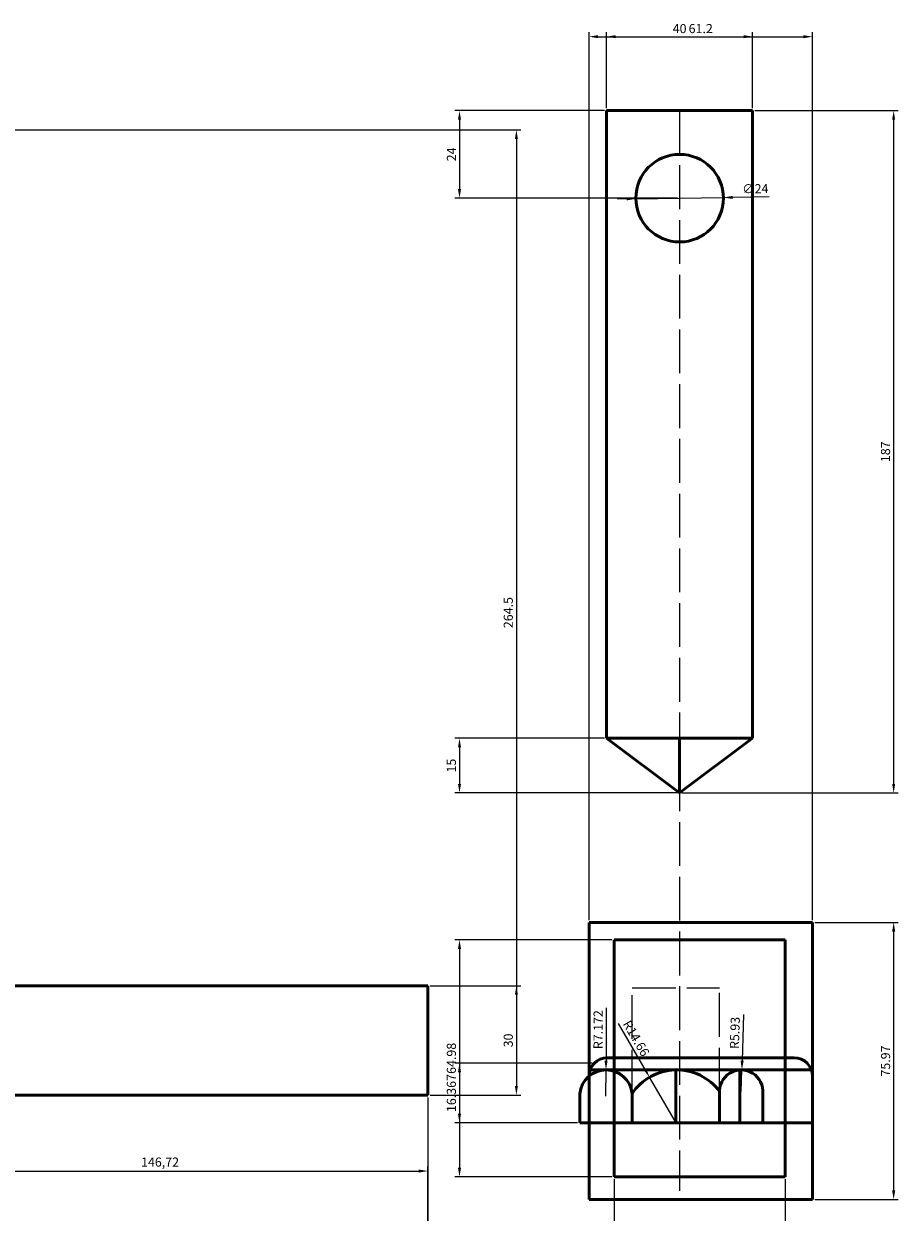
# Model space of a CAD drawing. Units: millimetres. Extents: x 921 to 2648, y 1390 to 2315.
# Tile 3 of 10: x 1184 to 1424, y 1882 to 2207. Entities that reach past the tile are written whole.
import ezdxf

# ---------------------------------------------------------------- set-up
doc = ezdxf.new("R2010")
doc.units = ezdxf.units.MM
doc.linetypes.add('ACAD_ISO02W100', pattern=[15, 12, -3])
for name, color, linetype, lineweight in [('M-DIMS', 2, 'Continuous', 25), ('M-HIDN', 4, 'ACAD_ISO02W100', 25), ('M-OUTL', 7, 'Continuous', 50)]:
    doc.layers.add(name, color=color, linetype=linetype, lineweight=lineweight)
doc.styles.get("Standard").update_dxf_attribs({"font": 'arial.ttf'})
doc.dimstyles.new('ISO-25', dxfattribs={"dimtxt": 2.5, "dimasz": 2.5, "dimexe": 1.25, "dimexo": 0.625, "dimtad": 1, "dimtxsty": 'Standard', "dimcen": 2.5, "dimadec": 0, "dimazin": 0, "dimtfac": 1, "dimtmove": 0, "dimatfit": 3, "dimfxl": 1, "dimarcsym": 0})

# ---------------------------------------------------------------- blocks, each defined once
blk = doc.blocks.new('*D18')
at = {"layer": 'Defpoints', "color": 0, "transparency": 16777216}
for p in [(1148.08, 1948.7), (1294.79, 1892.9), (1294.79, 1878.16)]:
    blk.add_point(p, dxfattribs=at)
at = {"layer": 'M-DIMS', "color": 0, "lineweight": -2, "transparency": 16777216}
for p, q in [((1148.08, 1948.07), (1148.08, 1891.65)), ((1150.58, 1892.9), (1292.29, 1892.9)), ((1294.79, 1878.78), (1294.79, 1894.15))]:
    blk.add_line(p, q, dxfattribs=at)
at = {"layer": 'M-DIMS', "color": 0, "transparency": 16777216}
for points in [[(1150.58, 1893.32), (1150.58, 1892.48), (1148.08, 1892.9)], [(1292.29, 1893.32), (1292.29, 1892.48), (1294.79, 1892.9)]]:
    blk.add_solid(points, dxfattribs=at)
at = {"layer": 'M-DIMS', "color": 0, "transparency": 16777216, "insert": (1221.43, 1895.03), "char_height": 2.5, "attachment_point": 5}
blk.add_mtext('146,72', dxfattribs=at)
blk = doc.blocks.new('*D24')
at = {"layer": 'Defpoints', "color": 0, "transparency": 16777216}
for p in [(1383.76, 2203.78), (1343.76, 2183.53), (1383.76, 2183.53)]:
    blk.add_point(p, dxfattribs=at)
at = {"layer": 'M-DIMS', "color": 0, "lineweight": -2, "transparency": 16777216}
for p, q in [((1343.76, 2184.15), (1343.76, 2205.03)), ((1346.26, 2203.78), (1381.26, 2203.78)), ((1383.76, 2184.15), (1383.76, 2205.03))]:
    blk.add_line(p, q, dxfattribs=at)
at = {"layer": 'M-DIMS', "color": 0, "transparency": 16777216}
for points in [[(1346.26, 2204.2), (1346.26, 2203.36), (1343.76, 2203.78)], [(1381.26, 2204.2), (1381.26, 2203.36), (1383.76, 2203.78)]]:
    blk.add_solid(points, dxfattribs=at)
at = {"layer": 'M-DIMS', "color": 0, "transparency": 16777216, "insert": (1363.76, 2205.68), "char_height": 2.5, "attachment_point": 5}
blk.add_mtext('40', dxfattribs=at)
blk = doc.blocks.new('*D25')
at = {"layer": 'Defpoints', "color": 0, "transparency": 16777216}
for p in [(1383.76, 2183.53), (1363.76, 1996.51), (1422.39, 1996.51)]:
    blk.add_point(p, dxfattribs=at)
at = {"layer": 'M-DIMS', "color": 0, "lineweight": -2, "transparency": 16777216}
for p, q in [((1384.39, 2183.53), (1423.64, 2183.53)), ((1422.39, 2181.03), (1422.39, 1999.01)), ((1364.39, 1996.51), (1423.64, 1996.51))]:
    blk.add_line(p, q, dxfattribs=at)
at = {"layer": 'M-DIMS', "color": 0, "transparency": 16777216}
for points in [[(1421.97, 2181.03), (1422.81, 2181.03), (1422.39, 2183.53)], [(1421.97, 1999.01), (1422.81, 1999.01), (1422.39, 1996.51)]]:
    blk.add_solid(points, dxfattribs=at)
at = {"layer": 'M-DIMS', "color": 0, "transparency": 16777216, "insert": (1420.49, 2090.02), "char_height": 2.5, "attachment_point": 5, "rotation": 90}
blk.add_mtext('187', dxfattribs=at)
blk = doc.blocks.new('*D45')
at = {"layer": 'Defpoints', "color": 0, "transparency": 16777216}
for p in [(1294.79, 1943.7), (1294.79, 1913.7), (1319.04, 1913.7)]:
    blk.add_point(p, dxfattribs=at)
at = {"layer": 'M-DIMS', "color": 0, "lineweight": -2, "transparency": 16777216}
for p, q in [((1295.42, 1943.7), (1320.29, 1943.7)), ((1319.04, 1941.2), (1319.04, 1916.2)), ((1295.42, 1913.7), (1320.29, 1913.7))]:
    blk.add_line(p, q, dxfattribs=at)
at = {"layer": 'M-DIMS', "color": 0, "transparency": 16777216}
for points in [[(1318.63, 1941.2), (1319.46, 1941.2), (1319.04, 1943.7)], [(1318.63, 1916.2), (1319.46, 1916.2), (1319.04, 1913.7)]]:
    blk.add_solid(points, dxfattribs=at)
at = {"layer": 'M-DIMS', "color": 0, "transparency": 16777216, "insert": (1317.14, 1928.7), "char_height": 2.5, "attachment_point": 5, "rotation": 90}
blk.add_mtext('30', dxfattribs=at)
blk = doc.blocks.new('*D46')
at = {"layer": 'Defpoints', "color": 0, "transparency": 16777216}
for p in [(1148.08, 2178.21), (1294.79, 1913.7), (1319.04, 1913.7)]:
    blk.add_point(p, dxfattribs=at)
at = {"layer": 'M-DIMS', "color": 0, "lineweight": -2, "transparency": 16777216}
for p, q in [((1148.7, 2178.21), (1320.29, 2178.21)), ((1319.04, 2175.71), (1319.04, 1916.2)), ((1295.42, 1913.7), (1320.29, 1913.7))]:
    blk.add_line(p, q, dxfattribs=at)
at = {"layer": 'M-DIMS', "color": 0, "transparency": 16777216}
for points in [[(1318.63, 2175.71), (1319.46, 2175.71), (1319.04, 2178.21)], [(1318.63, 1916.2), (1319.46, 1916.2), (1319.04, 1913.7)]]:
    blk.add_solid(points, dxfattribs=at)
at = {"layer": 'M-DIMS', "color": 0, "transparency": 16777216, "insert": (1317.14, 2045.95), "char_height": 2.5, "attachment_point": 5, "rotation": 90}
blk.add_mtext('264.5', dxfattribs=at)
blk = doc.blocks.new('*D49')
at = {"layer": 'Defpoints', "color": 0, "transparency": 16777216}
for p in [(950.61, 1913.7), (1294.79, 1913.7), (1294.79, 1705.98)]:
    blk.add_point(p, dxfattribs=at)
at = {"layer": 'M-DIMS', "color": 0, "lineweight": -2, "transparency": 16777216}
for p, q in [((950.61, 1913.07), (950.61, 1704.73)), ((1294.79, 1913.07), (1294.79, 1704.73)), ((953.11, 1705.98), (1292.29, 1705.98))]:
    blk.add_line(p, q, dxfattribs=at)
at = {"layer": 'M-DIMS', "color": 0, "transparency": 16777216}
for points in [[(953.11, 1706.4), (953.11, 1705.56), (950.61, 1705.98)], [(1292.29, 1706.4), (1292.29, 1705.56), (1294.79, 1705.98)]]:
    blk.add_solid(points, dxfattribs=at)
at = {"layer": 'M-DIMS', "color": 0, "transparency": 16777216, "insert": (1122.7, 1707.88), "char_height": 2.5, "attachment_point": 5}
blk.add_mtext('344.2', dxfattribs=at)
blk = doc.blocks.new('*D54')
at = {"layer": 'Defpoints', "color": 0, "transparency": 16777216}
for p in [(1343.76, 2183.53), (1303.46, 2159.53), (1363.76, 2159.53)]:
    blk.add_point(p, dxfattribs=at)
at = {"layer": 'M-DIMS', "color": 0, "lineweight": -2, "transparency": 16777216}
for p, q in [((1343.14, 2183.53), (1302.21, 2183.53)), ((1303.46, 2181.03), (1303.46, 2162.03)), ((1363.14, 2159.53), (1302.21, 2159.53))]:
    blk.add_line(p, q, dxfattribs=at)
at = {"layer": 'M-DIMS', "color": 0, "transparency": 16777216}
for points in [[(1303.04, 2181.03), (1303.88, 2181.03), (1303.46, 2183.53)], [(1303.04, 2162.03), (1303.88, 2162.03), (1303.46, 2159.53)]]:
    blk.add_solid(points, dxfattribs=at)
at = {"layer": 'M-DIMS', "color": 0, "transparency": 16777216, "insert": (1301.58, 2171.53), "char_height": 2.5, "attachment_point": 5, "rotation": 90}
blk.add_mtext('24', dxfattribs=at)
blk = doc.blocks.new('*D55')
at = {"layer": 'Defpoints', "color": 0, "transparency": 16777216}
for p in [(1343.76, 2011.51), (1303.46, 1996.51), (1363.76, 1996.51)]:
    blk.add_point(p, dxfattribs=at)
at = {"layer": 'M-DIMS', "color": 0, "lineweight": -2, "transparency": 16777216}
for p, q in [((1343.14, 2011.51), (1302.21, 2011.51)), ((1303.46, 2009.01), (1303.46, 1999.01)), ((1363.14, 1996.51), (1302.21, 1996.51))]:
    blk.add_line(p, q, dxfattribs=at)
at = {"layer": 'M-DIMS', "color": 0, "transparency": 16777216}
for points in [[(1303.04, 2009.01), (1303.88, 2009.01), (1303.46, 2011.51)], [(1303.04, 1999.01), (1303.88, 1999.01), (1303.46, 1996.51)]]:
    blk.add_solid(points, dxfattribs=at)
at = {"layer": 'M-DIMS', "color": 0, "transparency": 16777216, "insert": (1301.56, 2004.01), "char_height": 2.5, "attachment_point": 5, "rotation": 90}
blk.add_mtext('15', dxfattribs=at)
blk = doc.blocks.new('*D56')
at = {"layer": 'Defpoints', "color": 0, "transparency": 16777216}
for p in [(1400.14, 2203.78), (1338.94, 1961.04), (1400.14, 1961.04)]:
    blk.add_point(p, dxfattribs=at)
at = {"layer": 'M-DIMS', "color": 0, "lineweight": -2, "transparency": 16777216}
for p, q in [((1338.94, 1961.66), (1338.94, 2205.03)), ((1341.44, 2203.78), (1397.64, 2203.78)), ((1400.14, 1961.66), (1400.14, 2205.03))]:
    blk.add_line(p, q, dxfattribs=at)
at = {"layer": 'M-DIMS', "color": 0, "transparency": 16777216}
for points in [[(1341.44, 2204.2), (1341.44, 2203.36), (1338.94, 2203.78)], [(1397.64, 2204.2), (1397.64, 2203.36), (1400.14, 2203.78)]]:
    blk.add_solid(points, dxfattribs=at)
at = {"layer": 'M-DIMS', "color": 0, "transparency": 16777216, "insert": (1369.54, 2205.68), "char_height": 2.5, "attachment_point": 5}
blk.add_mtext('61.2', dxfattribs=at)
blk = doc.blocks.new('*D57')
at = {"layer": 'Defpoints', "color": 0, "transparency": 16777216}
for p in [(1400.14, 1961.04), (1400.14, 1885.07), (1422.39, 1885.07)]:
    blk.add_point(p, dxfattribs=at)
at = {"layer": 'M-DIMS', "color": 0, "lineweight": -2, "transparency": 16777216}
for p, q in [((1400.76, 1961.04), (1423.64, 1961.04)), ((1422.39, 1958.54), (1422.39, 1887.57)), ((1400.76, 1885.07), (1423.64, 1885.07))]:
    blk.add_line(p, q, dxfattribs=at)
at = {"layer": 'M-DIMS', "color": 0, "transparency": 16777216}
for points in [[(1421.97, 1958.54), (1422.81, 1958.54), (1422.39, 1961.04)], [(1421.97, 1887.57), (1422.81, 1887.57), (1422.39, 1885.07)]]:
    blk.add_solid(points, dxfattribs=at)
at = {"layer": 'M-DIMS', "color": 0, "transparency": 16777216, "insert": (1420.49, 1923.05), "char_height": 2.5, "attachment_point": 5, "rotation": 90}
blk.add_mtext('75.97', dxfattribs=at)
blk = doc.blocks.new('*D58')
at = {"layer": 'Defpoints', "color": 0, "transparency": 16777216}
for p in [(1345.83, 1891.3), (1392.63, 1891.3), (1392.63, 1779.85)]:
    blk.add_point(p, dxfattribs=at)
at = {"layer": 'M-DIMS', "color": 0, "lineweight": -2, "transparency": 16777216}
for p, q in [((1345.83, 1890.67), (1345.83, 1778.6)), ((1392.63, 1890.67), (1392.63, 1778.6)), ((1348.33, 1779.85), (1390.13, 1779.85))]:
    blk.add_line(p, q, dxfattribs=at)
at = {"layer": 'M-DIMS', "color": 0, "transparency": 16777216}
for points in [[(1348.33, 1780.27), (1348.33, 1779.44), (1345.83, 1779.85)], [(1390.13, 1780.27), (1390.13, 1779.44), (1392.63, 1779.85)]]:
    blk.add_solid(points, dxfattribs=at)
at = {"layer": 'M-DIMS', "color": 0, "transparency": 16777216, "insert": (1369.23, 1781.76), "char_height": 2.5, "attachment_point": 5}
blk.add_mtext('46.805', dxfattribs=at)
blk = doc.blocks.new('*D59')
at = {"layer": 'Defpoints', "color": 0, "transparency": 16777216}
for p in [(1345.83, 1956.28), (1303.46, 1891.3), (1345.83, 1891.3)]:
    blk.add_point(p, dxfattribs=at)
at = {"layer": 'M-DIMS', "color": 0, "lineweight": -2, "transparency": 16777216}
for p, q in [((1345.2, 1956.28), (1302.21, 1956.28)), ((1303.46, 1953.78), (1303.46, 1893.8)), ((1345.2, 1891.3), (1302.21, 1891.3))]:
    blk.add_line(p, q, dxfattribs=at)
at = {"layer": 'M-DIMS', "color": 0, "transparency": 16777216}
for points in [[(1303.04, 1953.78), (1303.88, 1953.78), (1303.46, 1956.28)], [(1303.04, 1893.8), (1303.88, 1893.8), (1303.46, 1891.3)]]:
    blk.add_solid(points, dxfattribs=at)
at = {"layer": 'M-DIMS', "color": 0, "transparency": 16777216, "insert": (1301.56, 1923.79), "char_height": 2.5, "attachment_point": 5, "rotation": 90}
blk.add_mtext('64.98', dxfattribs=at)
blk = doc.blocks.new('*D60')
at = {"layer": 'Defpoints', "color": 0, "transparency": 16777216}
for p in [(1340.4, 1922.46), (1303.46, 1906.09), (1336.44, 1906.09)]:
    blk.add_point(p, dxfattribs=at)
at = {"layer": 'M-DIMS', "color": 0, "lineweight": -2, "transparency": 16777216}
for p, q in [((1339.78, 1922.46), (1302.21, 1922.46)), ((1303.46, 1919.96), (1303.46, 1908.59)), ((1335.82, 1906.09), (1302.21, 1906.09))]:
    blk.add_line(p, q, dxfattribs=at)
at = {"layer": 'M-DIMS', "color": 0, "transparency": 16777216}
for points in [[(1303.04, 1919.96), (1303.88, 1919.96), (1303.46, 1922.46)], [(1303.04, 1908.59), (1303.88, 1908.59), (1303.46, 1906.09)]]:
    blk.add_solid(points, dxfattribs=at)
at = {"layer": 'M-DIMS', "color": 0, "transparency": 16777216, "insert": (1301.56, 1914.28), "char_height": 2.5, "attachment_point": 5, "rotation": 90}
blk.add_mtext('16.367', dxfattribs=at)
blk = doc.blocks.new('*D130')
at = {"layer": 'Defpoints', "color": 0, "transparency": 16777216}
for p in [(1375.76, 2159.7), (1351.76, 2159.36)]:
    blk.add_point(p, dxfattribs=at)
at = {"layer": 'M-DIMS', "color": 0, "lineweight": -2, "transparency": 16777216}
for p, q in [((1351.76, 2159.36), (1375.76, 2159.7)), ((1388.3, 2159.87), (1378.26, 2159.73)), ((1349.26, 2159.33), (1346.76, 2159.29))]:
    blk.add_line(p, q, dxfattribs=at)
at = {"layer": 'M-DIMS', "color": 0, "transparency": 16777216}
for points in [[(1349.26, 2159.74), (1349.27, 2158.91), (1351.76, 2159.36)], [(1378.25, 2160.15), (1378.27, 2159.32), (1375.76, 2159.7)]]:
    blk.add_solid(points, dxfattribs=at)
at = {"layer": 'M-DIMS', "color": 0, "transparency": 16777216, "insert": (1384.5, 2161.79), "char_height": 2.5, "attachment_point": 5, "rotation": 0.8039}
blk.add_mtext('∅24', dxfattribs=at)
blk = doc.blocks.new('*D131')
at = {"layer": 'Defpoints', "color": 0, "transparency": 16777216}
for p in [(1343.6, 1920.62), (1343.58, 1913.45)]:
    blk.add_point(p, dxfattribs=at)
at = {"layer": 'M-DIMS', "color": 0, "lineweight": -2, "transparency": 16777216}
for p, q in [((1343.64, 1937.67), (1343.61, 1923.12)), ((1343.58, 1913.45), (1343.6, 1920.62))]:
    blk.add_line(p, q, dxfattribs=at)
at = {"layer": 'M-DIMS', "color": 0, "transparency": 16777216}
blk.add_solid([(1343.19, 1923.12), (1344.02, 1923.12), (1343.6, 1920.62)], dxfattribs=at)
at = {"layer": 'M-DIMS', "color": 0, "transparency": 16777216, "insert": (1341.75, 1931.65), "char_height": 2.5, "attachment_point": 5, "rotation": 89.8664}
blk.add_mtext('R7.172', dxfattribs=at)
blk = doc.blocks.new('*D132')
at = {"layer": 'Defpoints', "color": 0, "transparency": 16777216}
for p in [(1355.52, 1918.61), (1362.93, 1905.96)]:
    blk.add_point(p, dxfattribs=at)
at = {"layer": 'M-DIMS', "color": 0, "lineweight": -2, "transparency": 16777216}
for p, q in [((1346.89, 1933.35), (1354.26, 1920.77)), ((1362.93, 1905.96), (1355.52, 1918.61))]:
    blk.add_line(p, q, dxfattribs=at)
at = {"layer": 'M-DIMS', "color": 0, "transparency": 16777216}
blk.add_solid([(1354.62, 1920.98), (1353.9, 1920.56), (1355.52, 1918.61)], dxfattribs=at)
at = {"layer": 'M-DIMS', "color": 0, "transparency": 16777216, "insert": (1351.58, 1929.1), "char_height": 2.5, "attachment_point": 5, "rotation": 300.3461}
blk.add_mtext('R14.66', dxfattribs=at)
blk = doc.blocks.new('*D133')
at = {"layer": 'Defpoints', "color": 0, "transparency": 16777216}
for p in [(1380.81, 1920.63), (1380.63, 1914.7)]:
    blk.add_point(p, dxfattribs=at)
at = {"layer": 'M-DIMS', "color": 0, "lineweight": -2, "transparency": 16777216}
for p, q in [((1381.27, 1935.76), (1380.88, 1923.13)), ((1380.63, 1914.7), (1380.81, 1920.63))]:
    blk.add_line(p, q, dxfattribs=at)
at = {"layer": 'M-DIMS', "color": 0, "transparency": 16777216}
blk.add_solid([(1380.47, 1923.14), (1381.3, 1923.12), (1380.81, 1920.63)], dxfattribs=at)
at = {"layer": 'M-DIMS', "color": 0, "transparency": 16777216, "insert": (1379.21, 1930.75), "char_height": 2.5, "attachment_point": 5, "rotation": 88.2471}
blk.add_mtext('R5.93', dxfattribs=at)

msp = doc.modelspace()

# ---------------------------------------------------------------- linework, layer by layer
at = {"layer": 'M-HIDN'}
for p, q in [((1363.7606, 2183.5297), (1363.7606, 1887.5032)), ((1350.7267, 1914.093), (1350.7267, 1943.1567)), ((1350.7267, 1943.1567), (1374.6954, 1943.1567)), ((1374.6954, 1914.7016), (1374.6954, 1943.1567))]:
    msp.add_line(p, q, dxfattribs=at)
at = {"layer": 'M-OUTL'}
for p, q in [((1343.7606, 2049.9042), (1343.7606, 2183.5297)), ((1343.7606, 2183.5297), (1383.7606, 2183.5297)), ((1383.7606, 2183.5297), (1383.7606, 2011.5146)), ((1343.7606, 2011.5146), (1343.7606, 2049.9042)), ((1383.7606, 2011.5146), (1343.7606, 2011.5146)), ((1343.7606, 2011.5146), (1363.7606, 1996.5146)), ((1363.7606, 2011.5146), (1363.7606, 1996.5146)), ((1363.7606, 1996.5146), (1383.7606, 2011.5146)), ((1338.9375, 1961.0383), (1400.1365, 1961.0383)), ((1338.9375, 1961.0383), (1338.9375, 1918.9245)), ((1400.1365, 1961.0383), (1400.1365, 1918.9245)), ((1345.8257, 1956.2798), (1392.6304, 1956.2798)), ((1345.8257, 1956.2798), (1345.8257, 1891.2986)), ((1392.6304, 1956.2798), (1392.6304, 1891.2986)), ((1294.7941, 1943.699), (1153.0755, 1943.699)), ((1294.7941, 1913.699), (1294.7941, 1943.699)), ((1343.9375, 1923.9245), (1395.1365, 1923.9245)), ((1343.5838, 1920.621), (1338.9375, 1920.621)), ((1338.9375, 1918.9245), (1338.9375, 1885.0696)), ((1343.5838, 1920.621), (1400.1365, 1920.621)), ((1362.7267, 1906.093), (1362.7267, 1920.621)), ((1380.2667, 1906.093), (1380.2667, 1920.621)), ((1400.1365, 1918.9245), (1400.1365, 1885.0696)), ((950.6135, 1913.699), (1294.7941, 1913.699)), ((1336.4409, 1914.093), (1336.4409, 1906.093)), ((1350.7267, 1914.093), (1350.7267, 1906.093)), ((1374.7267, 1906.093), (1374.7267, 1914.093)), ((1386.5245, 1914.093), (1386.5245, 1906.093)), ((1336.4409, 1906.093), (1400.1365, 1906.093)), ((1350.7267, 1906.093), (1362.7267, 1906.093)), ((1374.7267, 1906.093), (1380.2667, 1906.093)), ((1392.6304, 1891.2986), (1345.8257, 1891.2986)), ((1400.1365, 1885.0696), (1338.9375, 1885.0696))]:
    msp.add_line(p, q, dxfattribs=at)
msp.add_circle((1363.7606, 2159.5297), 12, dxfattribs=at)
for centre, radius, start, end in [((1343.9375, 1918.9245), 5, 90, 180), ((1395.1365, 1918.9245), 5, 0, 90), ((1343.5838, 1913.4491), 7.1719, 5.150903, 174.849097), ((1362.9252, 1905.9626), 14.6597, 36.592823, 146.316372), ((1380.6256, 1914.7016), 5.9302, 354.109194, 185.890806)]:
    msp.add_arc(centre, radius, start, end, dxfattribs=at)

# ---------------------------------------------------------------- dimensions: what is measured, and where the dimension line sits
at = {"layer": 'M-DIMS'}
for base, p1, p2, override, picture, middle in [((1400.1365, 2203.7797), (1338.9375, 1961.0383), (1400.1365, 1961.0383), {"dimdec": 1, "dimlfac": 1, "dimrnd": 0, "dimzin": 0, "dimdsep": 46, "dimlunit": 2}, '*D56', (1369.537, 2205.6811)), ((1383.7606, 2203.7797), (1343.7606, 2183.5297), (1383.7606, 2183.5297), {"dimdec": 0, "dimlfac": 1, "dimrnd": 0, "dimzin": 0, "dimdsep": 46, "dimlunit": 2}, '*D24', (1363.7606, 2205.6811)), ((1294.7941, 1892.9016), (1148.0755, 1948.699), (1294.7941, 1878.159), {"dimclrd": 0, "dimclre": 0, "dimclrt": 0}, '*D18', (1221.4348, 1895.029)), ((1294.7941, 1705.9795), (950.6135, 1913.699), (1294.7941, 1913.699), {"dimdec": 1, "dimlfac": 1, "dimrnd": 0, "dimzin": 0, "dimdsep": 46, "dimlunit": 2}, '*D49', (1122.7038, 1707.8818)), ((1392.6304, 1779.8536), (1345.8257, 1891.2986), (1392.6304, 1891.2986), {"dimdec": 3, "dimlfac": 1, "dimrnd": 0, "dimzin": 0, "dimdsep": 46, "dimlunit": 2}, '*D58', (1369.2281, 1781.7551))]:
    dim = msp.add_linear_dim(base=base, p1=p1, p2=p2, dimstyle='ISO-25', override=override, dxfattribs=at)
    dim.commit()
    dim.dimension.update_dxf_attribs({"geometry": picture, "text_midpoint": middle})
for base, p1, p2, override, picture, middle in [((1303.4605, 2159.5297), (1343.7606, 2183.5297), (1363.7606, 2159.5297), {"dimdec": 0, "dimlfac": 1, "dimrnd": 0, "dimzin": 0, "dimdsep": 46, "dimlunit": 2}, '*D54', (1301.5804, 2171.5297)), ((1422.3891, 1996.5146), (1383.7606, 2183.5297), (1363.7606, 1996.5146), {"dimdec": 0, "dimlfac": 1, "dimrnd": 0, "dimzin": 0, "dimdsep": 46, "dimlunit": 2}, '*D25', (1420.4877, 2090.0221)), ((1319.0441, 1913.699), (1148.0755, 2178.2093), (1294.7941, 1913.699), {"dimdec": 1, "dimlfac": 1, "dimrnd": 0, "dimzin": 0, "dimdsep": 46, "dimlunit": 2}, '*D46', (1317.1427, 2045.9541)), ((1303.4605, 1996.5146), (1343.7606, 2011.5146), (1363.7606, 1996.5146), {"dimdec": 0, "dimlfac": 1, "dimrnd": 0, "dimzin": 0, "dimdsep": 46, "dimlunit": 2}, '*D55', (1301.559, 2004.0146)), ((1422.3891, 1885.0696), (1400.1365, 1961.0383), (1400.1365, 1885.0696), {"dimdec": 2, "dimlfac": 1, "dimrnd": 0, "dimzin": 0, "dimdsep": 46, "dimlunit": 2}, '*D57', (1420.4877, 1923.0539)), ((1303.4605, 1891.2986), (1345.8257, 1956.2798), (1345.8257, 1891.2986), {"dimdec": 2, "dimlfac": 1, "dimrnd": 0, "dimzin": 0, "dimdsep": 46, "dimlunit": 2}, '*D59', (1301.559, 1923.7892)), ((1319.0441, 1913.699), (1294.7941, 1943.699), (1294.7941, 1913.699), {"dimdec": 0, "dimlfac": 1, "dimrnd": 0, "dimzin": 0, "dimdsep": 46, "dimlunit": 2}, '*D45', (1317.1419, 1928.699)), ((1303.4605, 1906.093), (1340.402, 1922.46), (1336.4409, 1906.093), {"dimdec": 3, "dimlfac": 1, "dimrnd": 0, "dimzin": 0, "dimdsep": 46, "dimlunit": 2}, '*D60', (1301.5582, 1914.2765))]:
    dim = msp.add_linear_dim(base=base, p1=p1, p2=p2, angle=90, dimstyle='ISO-25', override=override, dxfattribs=at)
    dim.commit()
    dim.dimension.update_dxf_attribs({"geometry": picture, "text_midpoint": middle})
dim = msp.add_diameter_dim_2p(p1=(1351.7618, 2159.3613), p2=(1375.7594, 2159.698), dimstyle='ISO-25', override={"dimdec": 0, "dimlfac": 1, "dimrnd": 0, "dimzin": 0, "dimdsep": 46, "dimlunit": 2}, dxfattribs=at)
dim.commit()
dim.dimension.update_dxf_attribs({"geometry": '*D130', "text_midpoint": (1384.529, 2159.8211)})
for center, mpoint, override, picture, middle in [((1343.5838, 1913.4491), (1343.6005, 1920.6209), {"dimdec": 3, "dimlfac": 1, "dimrnd": 0, "dimzin": 0, "dimdsep": 46, "dimlunit": 2}, '*D131', (1341.7461, 1931.6519)), ((1380.6256, 1914.7016), (1380.807, 1920.6291), {"dimdec": 2, "dimlfac": 1, "dimrnd": 0, "dimzin": 0, "dimdsep": 46, "dimlunit": 2}, '*D133', (1379.2136, 1930.7508)), ((1362.9252, 1905.9626), (1355.5188, 1918.6138), {"dimdec": 2, "dimlfac": 1, "dimrnd": 0, "dimzin": 0, "dimdsep": 46, "dimlunit": 2}, '*D132', (1351.5828, 1929.1006))]:
    dim = msp.add_radius_dim(center=center, mpoint=mpoint, dimstyle='ISO-25', override=override, dxfattribs=at)
    dim.commit()
    dim.dimension.update_dxf_attribs({"geometry": picture, "text_midpoint": middle})

doc.saveas('drawing.dxf')
